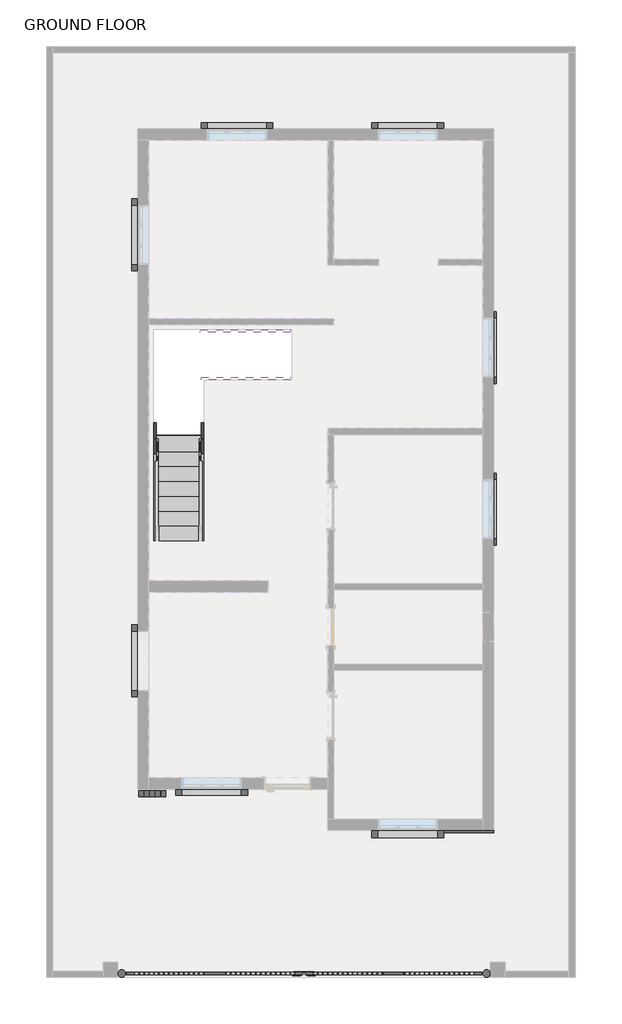
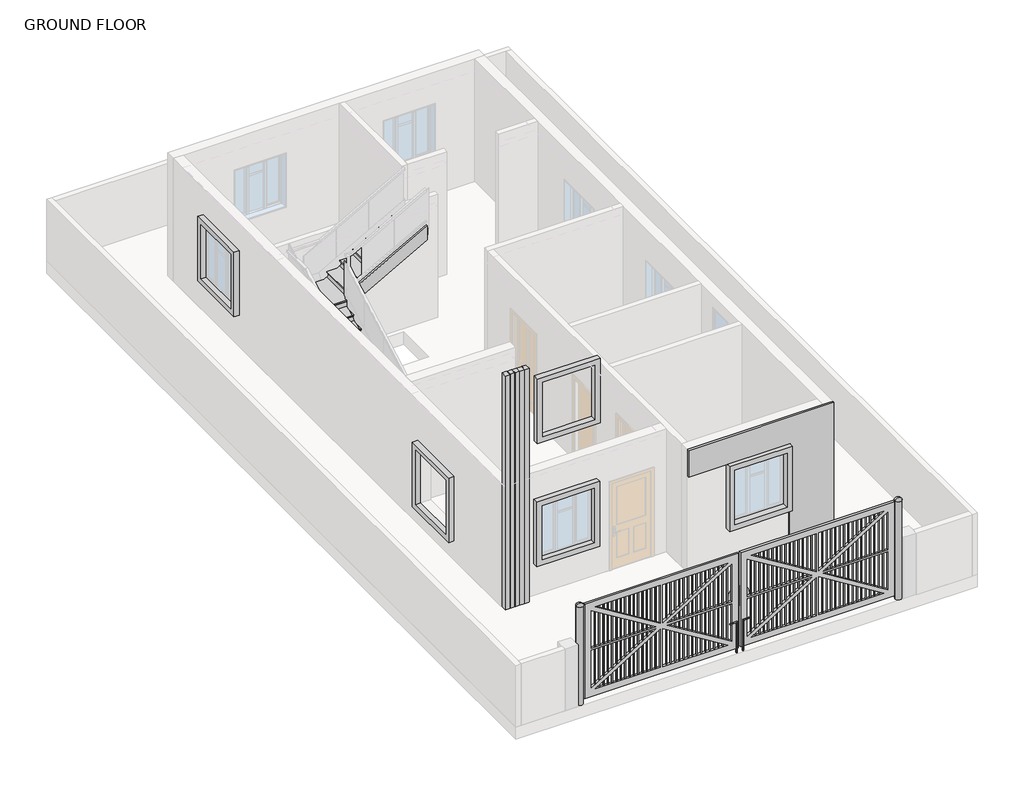
# One storey, part 4 of 4: 10 proxies, 4 members, 1 stair flight.
"""IFC4 building model written with IfcOpenShell, lengths in millimetres."""

from ifc_helpers import new_model, si_unit, frame, origin, place, context, project, spatial, polyline, outline, extrude, transform, mapped, element, save
from components import double_metal_gate_10830_double_metal_gate_10830_28153ce0, generic_models_11_generic_models_11_47c1f207, generic_models_12_generic_models_12_bd71d687, generic_models_14_generic_models_14_97bd1c4e, generic_models_18_generic_models_18_2803ece5, generic_models_2_generic_models_2_8f6bc761, generic_models_8_generic_models_5_f34dc4a4, generic_models_9_generic_models_9_4a2afa81, stair_flight_5b7f780d

model = new_model("IFC4")

# Units and contexts
model_context = context("Model", 3, world=origin())
ifc_project = project(units=[si_unit("LENGTHUNIT", "METRE", prefix="MILLI")], contexts=[model_context])

# Site, building, storey
site = spatial("IfcSite", under=ifc_project)
building = spatial("IfcBuilding", under=site)
storey = spatial("IfcBuildingStorey", under=building, Name="GROUND FLOOR", Elevation=304.8)

# Proxies
placement = place(None, origin())
double_metal_gate_10830_double_metal_gate_10830_shape = double_metal_gate_10830_double_metal_gate_10830_28153ce0(model_context)
element("IfcBuildingElementProxy", 1, Name="DOUBLE_METAL_GATE_10830 : DOUBLE_METAL_GATE_10830", ObjectType="DOUBLE_METAL_GATE_10830 : DOUBLE_METAL_GATE_10830", at=placement, inside=storey, context=model_context, shape_type="MappedRepresentation", body=[
    mapped(double_metal_gate_10830_double_metal_gate_10830_shape, transform((-5530.9607439, -9574.3210084, 304.8), x_axis=(1.0, 0.0, 0.0), y_axis=(0.0, 1.0, 0.0), z_axis=(0.0, 0.0, 1.0))),
])
generic_models_11_generic_models_11_shape = generic_models_11_generic_models_11_47c1f207(model_context)
element("IfcBuildingElementProxy", 2, Name="Generic Models 11 : Generic Models 11", ObjectType="Generic Models 11 : Generic Models 11", at=placement, inside=storey, context=model_context, shape_type="MappedRepresentation", body=[
    mapped(generic_models_11_generic_models_11_shape, transform((0.0, 0.0, 0.0), x_axis=(1.0, 0.0, 0.0), y_axis=(0.0, 1.0, 0.0), z_axis=(0.0, 0.0, 1.0))),
])
generic_models_12_generic_models_12_shape = generic_models_12_generic_models_12_bd71d687(model_context)
element("IfcBuildingElementProxy", 3, Name="Generic Models 12 : Generic Models 12", ObjectType="Generic Models 12 : Generic Models 12", at=placement, inside=storey, context=model_context, shape_type="MappedRepresentation", body=[
    mapped(generic_models_12_generic_models_12_shape, transform((0.0, 0.0, 0.0), x_axis=(1.0, 0.0, 0.0), y_axis=(0.0, 1.0, 0.0), z_axis=(0.0, 0.0, 1.0))),
])
generic_models_14_generic_models_14_shape = generic_models_14_generic_models_14_97bd1c4e(model_context)
element("IfcBuildingElementProxy", 4, Name="Generic Models 16 : Generic Models 14", ObjectType="Generic Models 16 : Generic Models 14", at=placement, inside=storey, context=model_context, shape_type="MappedRepresentation", body=[
    mapped(generic_models_14_generic_models_14_shape, transform((-38.1, 0.0, -3048.0), x_axis=(1.0, 0.0, 0.0), y_axis=(0.0, 1.0, 0.0), z_axis=(0.0, 0.0, 1.0))),
])
element("IfcBuildingElementProxy", 5, Name="Generic Models 17 : Generic Models 14", ObjectType="Generic Models 17 : Generic Models 14", at=placement, inside=storey, context=model_context, shape_type="MappedRepresentation", body=[
    mapped(generic_models_14_generic_models_14_shape, transform((-3531.39375, 0.0, -3048.0), x_axis=(1.0, 0.0, 0.0), y_axis=(0.0, 1.0, 0.0), z_axis=(0.0, 0.0, 1.0))),
])
generic_models_18_generic_models_18_shape = generic_models_18_generic_models_18_2803ece5(model_context)
element("IfcBuildingElementProxy", 6, Name="Generic Models 18 : Generic Models 18", ObjectType="Generic Models 18 : Generic Models 18", at=placement, inside=storey, context=model_context, shape_type="MappedRepresentation", body=[
    mapped(generic_models_18_generic_models_18_shape, transform((0.0, 0.0, 0.0), x_axis=(1.0, 0.0, 0.0), y_axis=(0.0, 1.0, 0.0), z_axis=(0.0, 0.0, 1.0))),
])
element("IfcBuildingElementProxy", 7, Name="Generic Models 19 : Generic Models 18", ObjectType="Generic Models 19 : Generic Models 18", at=placement, inside=storey, context=model_context, shape_type="MappedRepresentation", body=[
    mapped(generic_models_18_generic_models_18_shape, transform((0.0, -8719.3615197, -304.8), x_axis=(1.0, 0.0, 0.0), y_axis=(0.0, 1.0, 0.0), z_axis=(0.0, 0.0, 1.0))),
])
generic_models_2_generic_models_2_shape = generic_models_2_generic_models_2_8f6bc761(model_context)
element("IfcBuildingElementProxy", 8, Name="Generic Models 2 : Generic Models 2", ObjectType="Generic Models 2 : Generic Models 2", at=placement, inside=storey, context=model_context, shape_type="MappedRepresentation", body=[
    mapped(generic_models_2_generic_models_2_shape, transform((0.0, 0.0, 0.0), x_axis=(1.0, 0.0, 0.0), y_axis=(0.0, 1.0, 0.0), z_axis=(0.0, 0.0, 1.0))),
])
generic_models_8_generic_models_5_shape = generic_models_8_generic_models_5_f34dc4a4(model_context)
element("IfcBuildingElementProxy", 9, Name="Generic Models 8 : Generic Models 5", ObjectType="Generic Models 8 : Generic Models 5", at=placement, inside=storey, context=model_context, shape_type="MappedRepresentation", body=[
    mapped(generic_models_8_generic_models_5_shape, transform((-6429.5772098, 0.0, 0.0), x_axis=(1.0, 0.0, 0.0), y_axis=(0.0, 1.0, 0.0), z_axis=(0.0, 0.0, 1.0))),
])
generic_models_9_generic_models_9_shape = generic_models_9_generic_models_9_4a2afa81(model_context)
element("IfcBuildingElementProxy", 10, Name="Generic Models 9 : Generic Models 9", ObjectType="Generic Models 9 : Generic Models 9", at=placement, inside=storey, context=model_context, shape_type="MappedRepresentation", body=[
    mapped(generic_models_9_generic_models_9_shape, transform((0.0, 0.0, 0.0), x_axis=(1.0, 0.0, 0.0), y_axis=(0.0, 1.0, 0.0), z_axis=(0.0, 0.0, 1.0))),
])

# Members
element("IfcMember", 11, ObjectType="Stringer - 2\" Width", at=placement, inside=storey, context=model_context, shape_type="SweptSolid", body=[
    extrude(outline(polyline([(-642.5827462, 304.8), (-642.5827462, 512.3983948), (2099.0297538, 2035.5164503), (2726.6513672, 2035.5164503), (-388.6382434, 304.8), (-642.5827462, 304.8)])), frame((-9367.9482439, 0.0, 0.0), z_axis=(1.0, 0.0, 0.0), x_axis=(0.0, 1.0, 0.0)), (0.0, 0.0, 1.0), 50.8),
])
element("IfcMember", 12, ObjectType="Stringer - 2\" Width", at=placement, inside=storey, context=model_context, shape_type="SweptSolid", body=[
    extrude(outline(polyline([(2534.3863873, -7791.5607439), (3211.7197207, -6572.3607439), (3560.3983948, -6572.3607439), (2534.3863873, -8419.1823573), (2534.3863873, -7791.5607439)])), frame((0.0, 3624.6172538, 0.0), z_axis=(0.0, 1.0, 0.0), x_axis=(0.0, 0.0, 1.0)), (0.0, 0.0, 1.0), 50.8),
])
element("IfcMember", 13, ObjectType="Stringer - 2\" Width", at=placement, inside=storey, context=model_context, shape_type="SweptSolid", body=[
    extrude(outline(polyline([(-642.5827462, 304.8), (-642.5827462, 512.3983948), (2659.4172538, 2346.8428392), (2659.4172538, 1998.1641651), (-388.6382434, 304.8), (-642.5827462, 304.8)])), frame((-8401.1607439, 0.0, 0.0), z_axis=(1.0, 0.0, 0.0), x_axis=(0.0, 1.0, 0.0)), (0.0, 0.0, 1.0), 50.8),
])
element("IfcMember", 14, ObjectType="Stringer - 2\" Width", at=placement, inside=storey, context=model_context, shape_type="SweptSolid", body=[
    extrude(outline(polyline([(2544.3983948, -8401.1607439), (2195.7197207, -8401.1607439), (3211.7197207, -6572.3607439), (3560.3983948, -6572.3607439), (2544.3983948, -8401.1607439)])), frame((0.0, 2659.4172538, 0.0), z_axis=(0.0, 1.0, 0.0), x_axis=(0.0, 0.0, 1.0)), (0.0, 0.0, 1.0), 50.8),
])

# Stair flight
stair_flight_shape = stair_flight_5b7f780d(model_context)
element("IfcStairFlight", 15, ObjectType="2\" Tread 1\" Nosing 1/4\" Riser", at=placement, inside=storey, context=model_context, shape_type="MappedRepresentation", body=[
    mapped(stair_flight_shape, transform((0.0, 0.0, 0.0), x_axis=(1.0, 0.0, 0.0), y_axis=(0.0, 1.0, 0.0), z_axis=(0.0, 0.0, 1.0))),
])

save(model, "model.ifc")

# Revit data of these elements
# Type "DOUBLE_METAL_GATE_10830 : DOUBLE_METAL_GATE_10830"
#   WIDTH [instance default] = 24' - 0"
#   Default Elevation = 0
#   Assembly Code = ""
# Element 1 (IfcBuildingElementProxy, "DOUBLE_METAL_GATE_10830 : DOUBLE_METAL_GATE_10830")
#   WIDTH = 24' - 0"
#   Phase Created = New Construction
#   Materials on its faces: "Default"
# Element 2 (IfcBuildingElementProxy, "Generic Models 11 : Generic Models 11")
#   Phase Created = New Construction
#   Materials on its faces: "CLADDING WALL MATERIAL"
# Element 3 (IfcBuildingElementProxy, "Generic Models 12 : Generic Models 12")
#   Phase Created = New Construction
#   Materials on its faces: "BLACK"
# Element 4 (IfcBuildingElementProxy, "Generic Models 16 : Generic Models 14")
#   Phase Created = New Construction
#   Materials on its faces: "BLACK"
# Element 5 (IfcBuildingElementProxy, "Generic Models 17 : Generic Models 14")
#   Phase Created = New Construction
#   Materials on its faces: "BLACK"
# Element 6 (IfcBuildingElementProxy, "Generic Models 18 : Generic Models 18")
#   Phase Created = New Construction
#   Materials on its faces: "BLACK"
# Element 7 (IfcBuildingElementProxy, "Generic Models 19 : Generic Models 18")
#   Phase Created = New Construction
#   Materials on its faces: "BLACK"
# Element 8 (IfcBuildingElementProxy, "Generic Models 2 : Generic Models 2")
#   Phase Created = New Construction
#   Materials on its faces: "BLACK"
# Element 9 (IfcBuildingElementProxy, "Generic Models 8 : Generic Models 5")
#   Phase Created = New Construction
# Element 10 (IfcBuildingElementProxy, "Generic Models 9 : Generic Models 9")
#   Phase Created = New Construction
#   Materials on its faces: "BLACK"
# Element 11 (IfcMember, "Stringer - 2\" Width")
#   Phase Created = New Construction
# Elements 12, 13, 14 (IfcMember, "Stringer - 2\" Width")
#   Phase Created = New Construction
#   Materials on its faces: "BLACK"
# Element 15 (IfcStairFlight, "2\" Tread 1\" Nosing 1/4\" Riser")
#   Phase Created = New Construction
#   Materials on its faces: "MARBLE PAINT"
# Materials
#   "Default": colour RGB 127 127 127, transparency 0, Cost = 0
#   "CLADDING WALL MATERIAL": class "Generic", colour RGB 120 120 120, transparency 0, Cost = 0
#   "BLACK": class "Generic", colour RGB 120 120 120, transparency 0, Cost = 0
#   "MARBLE PAINT": class "Generic", colour RGB 120 120 120, transparency 0, Cost = 0
